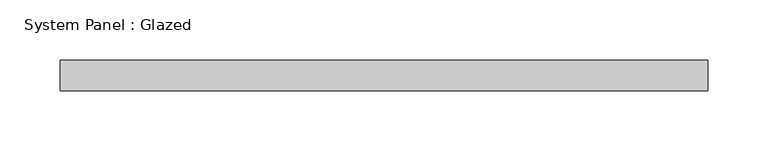
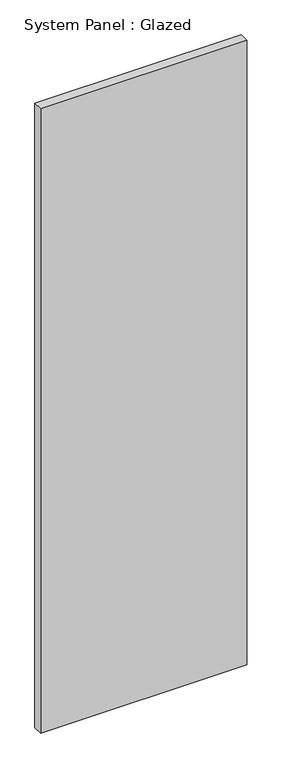
"""IFC4 building model written with IfcOpenShell, lengths in millimetres: plate geometry, System Panel : Glazed."""

from ifc_helpers import new_model, si_unit, origin, origin_with_axes, place, context, project, spatial, polyline, outline, extrude, source, transform, mapped, element, save


def system_panel_glazed_2339bcea(model_context):
    return source(origin(), model_context, "Body", "SweptSolid", [
        extrude(outline(polyline([(269.875, -44.45), (-269.875, -44.45), (-269.875, -19.05), (269.875, -19.05), (269.875, -44.45)])), origin_with_axes(), (0.0, 0.0, 1.0), 1727.2),
    ])


if __name__ == "__main__":
    model = new_model("IFC4")
    model_context = context("Model", 3, world=origin())
    ifc_project = project(units=[si_unit("LENGTHUNIT", "METRE", prefix="MILLI")], contexts=[model_context])
    site = spatial("IfcSite", under=ifc_project)
    building = spatial("IfcBuilding", under=site)
    placement = place(None, origin())
    system_panel_glazed_shape = system_panel_glazed_2339bcea(model_context)
    element("IfcPlate", 1, ObjectType="System Panel : Glazed", at=placement, inside=building, context=model_context, shape_type="MappedRepresentation", body=[
        mapped(system_panel_glazed_shape, transform((0.0, 0.0, 0.0), x_axis=(1.0, 0.0, 0.0), y_axis=(0.0, 1.0, 0.0), z_axis=(0.0, 0.0, 1.0))),
    ])
    save(model, "model.ifc")

# Revit data of these elements
# Type "System Panel : Glazed"
#   Construction Type Id = "GSP4R"
#   Analytic Construction = "1/8 in Pilkington single glazing"
#   Visual Light Transmittance = 0.9
#   Solar Heat Gain Coefficient = 0.86
#   Heat Transfer Coefficient (U) = 1.18115 BTU/(h·ft²·°F)
#   Define Thermal Properties by = 1
# Element 1 (IfcPlate, "System Panel : Glazed")
#   Materials on its faces: "Glass"
# Materials
#   "Glass": class "Glass", colour RGB 0 128 192, transparency 0.75, Description = "Soda Lime Glass", Cost = 0
